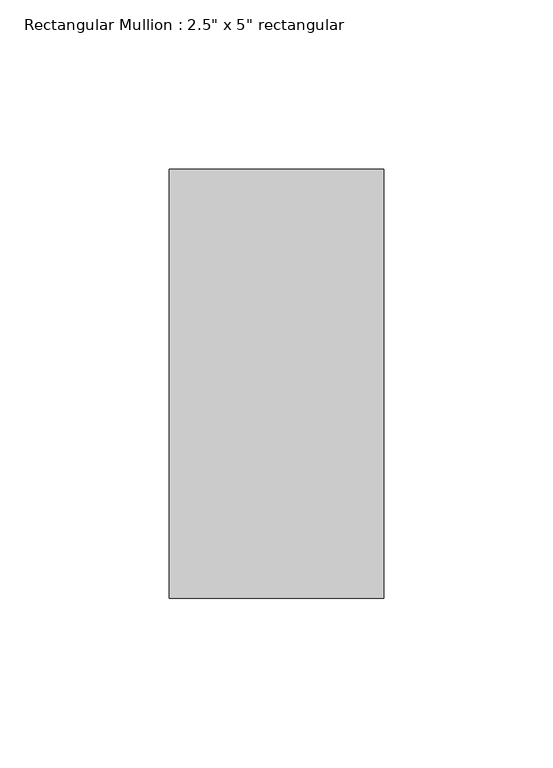
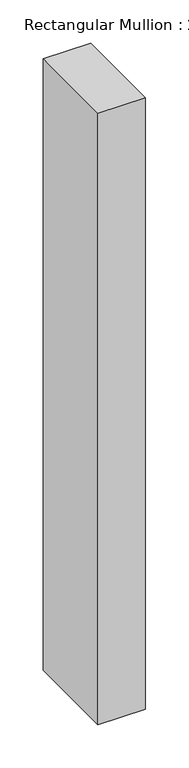
"""IFC4 building model written with IfcOpenShell, lengths in millimetres: member geometry."""

from ifc_helpers import new_model, si_unit, frame, origin, place, context, project, spatial, polyline, outline, extrude, source, transform, mapped, element, save


def member_96c05505(model_context):
    return source(origin(), model_context, "Body", "SweptSolid", [
        extrude(outline(polyline([(0.0, 63.5), (0.0, -63.5), (-63.5, -63.5), (-63.5, 63.5), (0.0, 63.5)])), frame((0.0, 0.0, -864.6440196), z_axis=(0.0, 0.0, 1.0), x_axis=(1.0, 0.0, 0.0)), (0.0, 0.0, 1.0), 864.6440196),
    ])


if __name__ == "__main__":
    model = new_model("IFC4")
    model_context = context("Model", 3, world=origin())
    ifc_project = project(units=[si_unit("LENGTHUNIT", "METRE", prefix="MILLI")], contexts=[model_context])
    site = spatial("IfcSite", under=ifc_project)
    building = spatial("IfcBuilding", under=site)
    placement = place(None, origin())
    member_shape = member_96c05505(model_context)
    element("IfcMember", 1, ObjectType="Rectangular Mullion : 2.5\" x 5\" rectangular", at=placement, inside=building, context=model_context, shape_type="MappedRepresentation", body=[
        mapped(member_shape, transform((0.0, 0.0, 0.0), x_axis=(1.0, 0.0, 0.0), y_axis=(0.0, 1.0, 0.0), z_axis=(0.0, 0.0, 1.0))),
    ])
    save(model, "model.ifc")

# Revit data of these elements
# Type "Rectangular Mullion : 2.5\" x 5\" rectangular"
#   built-in parameter 1007304 = 0.416667 (stored number, unit not read)
#   built-in parameter 1007301 = 0.104167 (stored number, unit not read)
#   built-in parameter 1007300 = 0.104167 (stored number, unit not read)
# Element 1 (IfcMember, "Rectangular Mullion : 2.5\" x 5\" rectangular")
#   Materials on its faces: "Aluminum"
# Materials
#   "Aluminum": class "Metal", colour RGB 247 247 247, transparency 0, Description = "Aluminum 6061", Cost = 0
